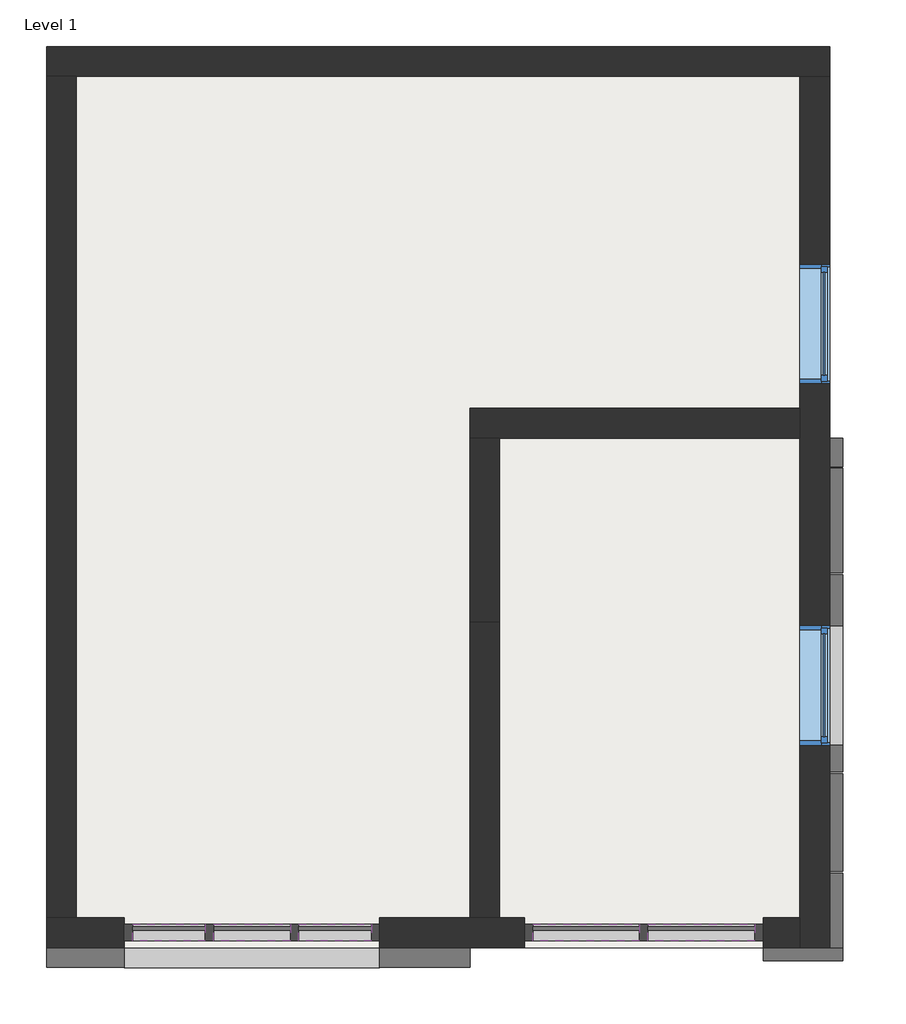
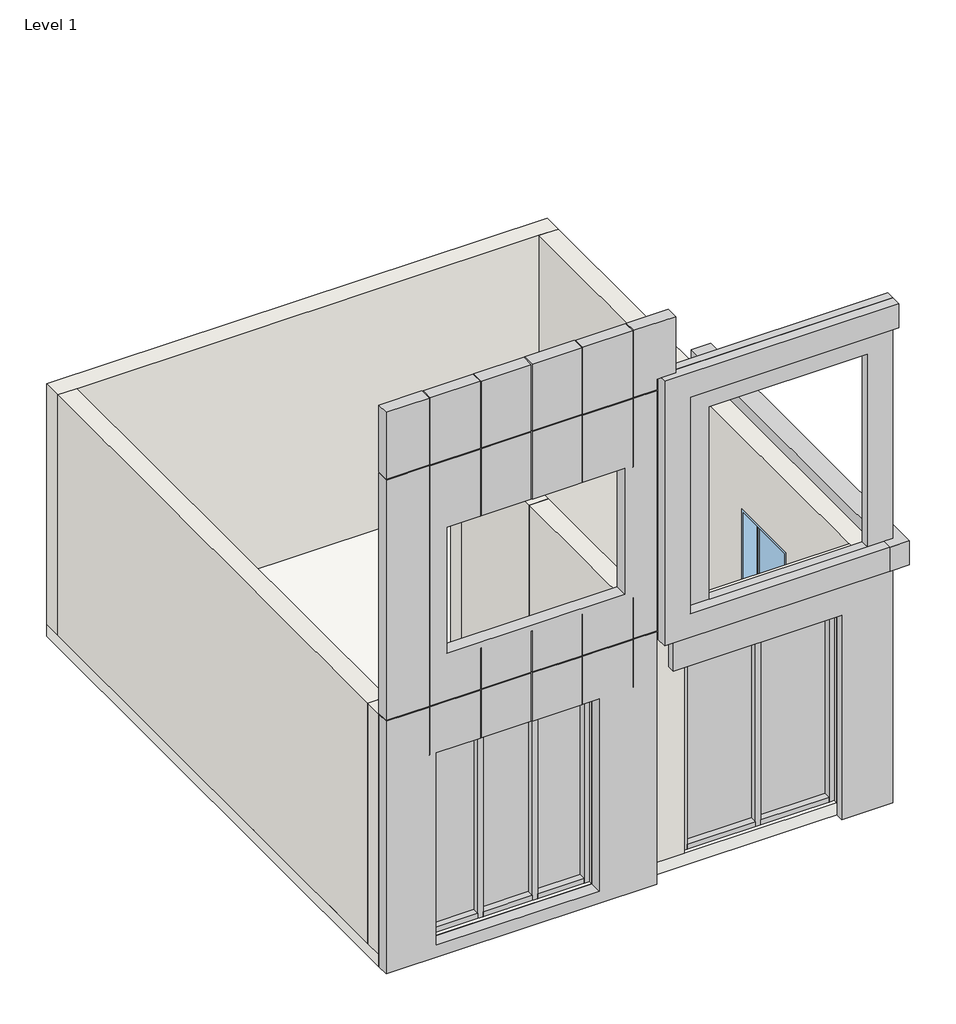
# One storey: 17 members, 7 walls, 5 plates, 2 windows, 1 proxy, 1 slab.
"""IFC4 building model written with IfcOpenShell, lengths in millimetres."""

from ifc_helpers import new_model, si_unit, frame, origin, origin_with_axes, place, context, project, spatial, polyline, outline, extrude, faceted_brep, transform, mapped, element, save
from components import generic_models_2_generic_models_2_1e037190, member_f0fea5a5, member_ee409385, member_c17f1be2, member_b26d3c89, member_9202991e, system_panel_glazed_061c0ed8, system_panel_glazed_2536b6f7, system_panel_glazed_348cf8e9, window_c1f32544, fixed_7_window_d95a62fe

model = new_model("IFC4")

# Units and contexts
model_context = context("Model", 3, world=origin())
ifc_project = project(units=[si_unit("LENGTHUNIT", "METRE", prefix="MILLI")], contexts=[model_context])

# Site, building, storey
site = spatial("IfcSite", under=ifc_project)
building = spatial("IfcBuilding", under=site)
storey = spatial("IfcBuildingStorey", under=building, Name="Level 1", Elevation=0.0)

# Proxy
placement = place(None, origin())
generic_models_2_generic_models_2_shape = generic_models_2_generic_models_2_1e037190(model_context)
element("IfcBuildingElementProxy", 1, Name="Generic Models 2 : Generic Models 2", ObjectType="Generic Models 2 : Generic Models 2", at=placement, inside=storey, context=model_context, shape_type="MappedRepresentation", body=[
    mapped(generic_models_2_generic_models_2_shape, transform((0.0, 0.0, 0.0), x_axis=(1.0, 0.0, 0.0), y_axis=(0.0, 1.0, 0.0), z_axis=(0.0, 0.0, 1.0))),
])

# Members
member_shape = member_f0fea5a5(model_context)
element("IfcMember", 2, ObjectType="Rectangular Mullion : 2.5\" x 5\" rectangular", at=placement, inside=storey, context=model_context, shape_type="MappedRepresentation", body=[
    mapped(member_shape, transform((-8698.6297584, 854.4262137, 0.0), x_axis=(1.0, 0.0, 0.0), y_axis=(0.0, -1.0, 0.0), z_axis=(0.0, 0.0, -1.0))),
])
element("IfcMember", 3, ObjectType="Rectangular Mullion : 2.5\" x 5\" rectangular", at=placement, inside=storey, context=model_context, shape_type="MappedRepresentation", body=[
    mapped(member_shape, transform((-12026.1620499, 854.4262137, 0.0), x_axis=(1.0, 0.0, 0.0), y_axis=(0.0, -1.0, 0.0), z_axis=(0.0, 0.0, -1.0))),
])
element("IfcMember", 4, ObjectType="Rectangular Mullion : 2.5\" x 5\" rectangular", at=placement, inside=storey, context=model_context, shape_type="MappedRepresentation", body=[
    mapped(member_shape, transform((-11374.2287168, 854.4262137, 0.0), x_axis=(1.0, 0.0, 0.0), y_axis=(0.0, -1.0, 0.0), z_axis=(0.0, 0.0, -1.0))),
])
member_2_shape = member_ee409385(model_context)
element("IfcMember", 5, ObjectType="Rectangular Mullion : 2.5\" x 5\" rectangular", at=placement, inside=storey, context=model_context, shape_type="MappedRepresentation", body=[
    mapped(member_2_shape, transform((-7784.2297584, 854.4262137, 0.0), x_axis=(1.0, 0.0, 0.0), y_axis=(0.0, -1.0, 0.0), z_axis=(0.0, 0.0, -1.0))),
])
element("IfcMember", 6, ObjectType="Rectangular Mullion : 2.5\" x 5\" rectangular", at=placement, inside=storey, context=model_context, shape_type="MappedRepresentation", body=[
    mapped(member_2_shape, transform((-10722.2953834, 854.4262137, 0.0), x_axis=(1.0, 0.0, 0.0), y_axis=(0.0, -1.0, 0.0), z_axis=(0.0, 0.0, -1.0))),
])
element("IfcMember", 7, ObjectType="Rectangular Mullion : 2.5\" x 5\" rectangular", at=placement, inside=storey, context=model_context, shape_type="MappedRepresentation", body=[
    mapped(member_2_shape, transform((-9613.0297584, 854.4262137, 2438.4), x_axis=(-1.0, 0.0, 0.0), y_axis=(0.0, -1.0, 0.0), z_axis=(0.0, 0.0, 1.0))),
])
element("IfcMember", 8, ObjectType="Rectangular Mullion : 2.5\" x 5\" rectangular", at=placement, inside=storey, context=model_context, shape_type="MappedRepresentation", body=[
    mapped(member_2_shape, transform((-12678.0953834, 854.4262137, 2438.4), x_axis=(-1.0, 0.0, 0.0), y_axis=(0.0, -1.0, 0.0), z_axis=(0.0, 0.0, 1.0))),
])
member_3_shape = member_c17f1be2(model_context)
element("IfcMember", 9, ObjectType="Rectangular Mullion : 2.5\" x 5\" rectangular", at=placement, inside=storey, context=model_context, shape_type="MappedRepresentation", body=[
    mapped(member_3_shape, transform((-7847.7297584, 854.4262137, 2438.4), x_axis=(0.0, 0.0, 1.0), y_axis=(0.0, -1.0, 0.0), z_axis=(1.0, 0.0, 0.0))),
])
element("IfcMember", 10, ObjectType="Rectangular Mullion : 2.5\" x 5\" rectangular", at=placement, inside=storey, context=model_context, shape_type="MappedRepresentation", body=[
    mapped(member_3_shape, transform((-8730.3797584, 854.4262137, 2438.4), x_axis=(0.0, 0.0, 1.0), y_axis=(0.0, -1.0, 0.0), z_axis=(1.0, 0.0, 0.0))),
])
element("IfcMember", 11, ObjectType="Rectangular Mullion : 2.5\" x 5\" rectangular", at=placement, inside=storey, context=model_context, shape_type="MappedRepresentation", body=[
    mapped(member_3_shape, transform((-9549.5297584, 854.4262137, 0.0), x_axis=(0.0, 0.0, -1.0), y_axis=(0.0, -1.0, 0.0), z_axis=(-1.0, 0.0, 0.0))),
])
element("IfcMember", 12, ObjectType="Rectangular Mullion : 2.5\" x 5\" rectangular", at=placement, inside=storey, context=model_context, shape_type="MappedRepresentation", body=[
    mapped(member_3_shape, transform((-8666.8797584, 854.4262137, 0.0), x_axis=(0.0, 0.0, -1.0), y_axis=(0.0, -1.0, 0.0), z_axis=(-1.0, 0.0, 0.0))),
])
member_4_shape = member_b26d3c89(model_context)
element("IfcMember", 13, ObjectType="Rectangular Mullion : 2.5\" x 5\" rectangular", at=placement, inside=storey, context=model_context, shape_type="MappedRepresentation", body=[
    mapped(member_4_shape, transform((-10785.7953834, 854.4262137, 2438.4), x_axis=(0.0, 0.0, 1.0), y_axis=(0.0, -1.0, 0.0), z_axis=(1.0, 0.0, 0.0))),
])
element("IfcMember", 14, ObjectType="Rectangular Mullion : 2.5\" x 5\" rectangular", at=placement, inside=storey, context=model_context, shape_type="MappedRepresentation", body=[
    mapped(member_4_shape, transform((-12057.9120499, 854.4262137, 2438.4), x_axis=(0.0, 0.0, 1.0), y_axis=(0.0, -1.0, 0.0), z_axis=(1.0, 0.0, 0.0))),
])
element("IfcMember", 15, ObjectType="Rectangular Mullion : 2.5\" x 5\" rectangular", at=placement, inside=storey, context=model_context, shape_type="MappedRepresentation", body=[
    mapped(member_4_shape, transform((-12614.5953834, 854.4262137, 0.0), x_axis=(0.0, 0.0, -1.0), y_axis=(0.0, -1.0, 0.0), z_axis=(-1.0, 0.0, 0.0))),
])
element("IfcMember", 16, ObjectType="Rectangular Mullion : 2.5\" x 5\" rectangular", at=placement, inside=storey, context=model_context, shape_type="MappedRepresentation", body=[
    mapped(member_4_shape, transform((-11342.4787168, 854.4262137, 0.0), x_axis=(0.0, 0.0, -1.0), y_axis=(0.0, -1.0, 0.0), z_axis=(-1.0, 0.0, 0.0))),
])
member_5_shape = member_9202991e(model_context)
element("IfcMember", 17, ObjectType="Rectangular Mullion : 2.5\" x 5\" rectangular", at=placement, inside=storey, context=model_context, shape_type="MappedRepresentation", body=[
    mapped(member_5_shape, transform((-11994.4120499, 854.4262137, 0.0), x_axis=(0.0, 0.0, -1.0), y_axis=(0.0, -1.0, 0.0), z_axis=(-1.0, 0.0, 0.0))),
])
element("IfcMember", 18, ObjectType="Rectangular Mullion : 2.5\" x 5\" rectangular", at=placement, inside=storey, context=model_context, shape_type="MappedRepresentation", body=[
    mapped(member_5_shape, transform((-11405.9787168, 854.4262137, 2438.4), x_axis=(0.0, 0.0, 1.0), y_axis=(0.0, -1.0, 0.0), z_axis=(1.0, 0.0, 0.0))),
])

# Plates
system_panel_glazed_shape = system_panel_glazed_061c0ed8(model_context)
element("IfcPlate", 19, ObjectType="System Panel : Glazed", at=placement, inside=storey, context=model_context, shape_type="MappedRepresentation", body=[
    mapped(system_panel_glazed_shape, transform((-9139.9547584, 854.4262137, 63.5), x_axis=(1.0, 0.0, 0.0), y_axis=(0.0, 1.0, 0.0), z_axis=(0.0, 0.0, 1.0))),
])
element("IfcPlate", 20, ObjectType="System Panel : Glazed", at=placement, inside=storey, context=model_context, shape_type="MappedRepresentation", body=[
    mapped(system_panel_glazed_shape, transform((-8257.3047584, 854.4262137, 63.5), x_axis=(1.0, 0.0, 0.0), y_axis=(0.0, 1.0, 0.0), z_axis=(0.0, 0.0, 1.0))),
])
system_panel_glazed_2_shape = system_panel_glazed_2536b6f7(model_context)
element("IfcPlate", 21, ObjectType="System Panel : Glazed", at=placement, inside=storey, context=model_context, shape_type="MappedRepresentation", body=[
    mapped(system_panel_glazed_2_shape, transform((-12336.2537167, 854.4262137, 63.5), x_axis=(1.0, 0.0, 0.0), y_axis=(0.0, 1.0, 0.0), z_axis=(0.0, 0.0, 1.0))),
])
element("IfcPlate", 22, ObjectType="System Panel : Glazed", at=placement, inside=storey, context=model_context, shape_type="MappedRepresentation", body=[
    mapped(system_panel_glazed_2_shape, transform((-11064.1370501, 854.4262137, 63.5), x_axis=(1.0, 0.0, 0.0), y_axis=(0.0, 1.0, 0.0), z_axis=(0.0, 0.0, 1.0))),
])
system_panel_glazed_3_shape = system_panel_glazed_348cf8e9(model_context)
element("IfcPlate", 23, ObjectType="System Panel : Glazed", at=placement, inside=storey, context=model_context, shape_type="MappedRepresentation", body=[
    mapped(system_panel_glazed_3_shape, transform((-11700.1953834, 854.4262137, 63.5), x_axis=(1.0, 0.0, 0.0), y_axis=(0.0, 1.0, 0.0), z_axis=(0.0, 0.0, 1.0))),
])

# Slab
element("IfcSlab", 24, ObjectType="6\" floor", at=placement, inside=storey, context=model_context, shape_type="SweptSolid", body=[
    extrude(outline(polyline([(-7274.9953834, 7640.1262137), (-7274.9953834, 740.1262137), (-13274.9953834, 740.1262137), (-13274.9953834, 7640.1262137), (-7274.9953834, 7640.1262137)])), frame((0.0, 0.0, -152.4), z_axis=(0.0, 0.0, 1.0), x_axis=(1.0, 0.0, 0.0)), (0.0, 0.0, 1.0), 152.4),
])

# Walls
element("IfcWall", 25, ObjectType="9\" wall", at=placement, inside=storey, context=model_context, shape_type="Brep", body=[
    faceted_brep([(-13274.9953834, 7411.5262137, 0.0), (-13046.3953834, 7411.5262137, 0.0), (-7503.5953834, 7411.5262137, 0.0), (-7274.9953834, 7411.5262137, 0.0), (-7274.9953834, 7411.5262137, 3048.0), (-7503.5953834, 7411.5262137, 3048.0), (-13046.3953834, 7411.5262137, 3048.0), (-13274.9953834, 7411.5262137, 3048.0), (-13274.9953834, 7640.1262137, 0.0), (-13274.9953834, 7640.1262137, 3048.0), (-7274.9953834, 7640.1262137, 3048.0), (-7274.9953834, 7640.1262137, 0.0)], [[[0, 1, 2, 3, 4, 5, 6, 7]], [[8, 9, 10, 11]], [[3, 2, 1, 0, 8, 11]], [[7, 6, 5, 4, 10, 9]], [[4, 3, 11, 10]], [[0, 7, 9, 8]]]),
])
element("IfcWall", 26, ObjectType="9\" wall", at=placement, inside=storey, context=model_context, shape_type="Brep", body=[
    faceted_brep([(-7503.5953834, 740.1262137, 3048.0), (-7503.5953834, 968.7262137, 3048.0), (-7503.5953834, 4640.1176199, 3048.0), (-7503.5953834, 4868.7176199, 3048.0), (-7503.5953834, 7411.5262137, 3048.0), (-7503.5953834, 7411.5262137, 0.0), (-7503.5953834, 4868.7176199, 0.0), (-7503.5953834, 4640.1176199, 0.0), (-7503.5953834, 3205.0176199, 0.0), (-7503.5953834, 3205.0176199, 2133.6), (-7503.5953834, 2290.6176199, 2133.6), (-7503.5953834, 2290.6176199, 0.0), (-7503.5953834, 968.7262137, 0.0), (-7503.5953834, 740.1262137, 0.0), (-7503.5953834, 5059.2176199, 2133.6), (-7503.5953834, 5059.2176199, 914.4), (-7503.5953834, 5973.6176199, 914.4), (-7503.5953834, 5973.6176199, 2133.6), (-7274.9953834, 7411.5262137, 3048.0), (-7274.9953834, 740.1262137, 3048.0), (-7274.9953834, 740.1262137, 0.0), (-7274.9953834, 2290.6176199, 0.0), (-7274.9953834, 2290.6176199, 2133.6), (-7274.9953834, 3205.0176199, 2133.6), (-7274.9953834, 3205.0176199, 0.0), (-7274.9953834, 7411.5262137, 0.0), (-7274.9953834, 5059.2176199, 2133.6), (-7274.9953834, 5973.6176199, 2133.6), (-7274.9953834, 5973.6176199, 914.4), (-7274.9953834, 5059.2176199, 914.4)], [[[0, 1, 2, 3, 4, 5, 6, 7, 8, 9, 10, 11, 12, 13], [14, 15, 16, 17]], [[18, 19, 20, 21, 22, 23, 24, 25], [26, 27, 28, 29]], [[5, 25, 24, 8, 7, 6]], [[20, 13, 12, 11, 21]], [[4, 3, 2, 1, 0, 19, 18]], [[5, 4, 18, 25]], [[0, 13, 20, 19]], [[15, 14, 26, 29]], [[16, 15, 29, 28]], [[17, 16, 28, 27]], [[14, 17, 27, 26]], [[10, 22, 21, 11]], [[23, 9, 8, 24]], [[22, 10, 9, 23]]]),
])
element("IfcWall", 27, ObjectType="9\" wall", at=placement, inside=storey, context=model_context, shape_type="Brep", body=[
    faceted_brep([(-13274.9953834, 968.7262137, 3048.0), (-13046.3953834, 968.7262137, 3048.0), (-10032.1297584, 968.7262137, 3048.0), (-9803.5297584, 968.7262137, 3048.0), (-7503.5953834, 968.7262137, 3048.0), (-7503.5953834, 968.7262137, 0.0), (-7784.2297584, 968.7262137, 0.0), (-7784.2297584, 968.7262137, 2438.4), (-9613.0297584, 968.7262137, 2438.4), (-9613.0297584, 968.7262137, 0.0), (-9803.5297584, 968.7262137, 0.0), (-10032.1297584, 968.7262137, 0.0), (-10722.2953834, 968.7262137, 0.0), (-10722.2953834, 968.7262137, 2438.4), (-12678.0953834, 968.7262137, 2438.4), (-12678.0953834, 968.7262137, 0.0), (-13046.3953834, 968.7262137, 0.0), (-13274.9953834, 968.7262137, 0.0), (-7503.5953834, 740.1262137, 3048.0), (-13274.9953834, 740.1262137, 3048.0), (-13274.9953834, 740.1262137, 0.0), (-12678.0953834, 740.1262137, 0.0), (-12678.0953834, 740.1262137, 2438.4), (-10722.2953834, 740.1262137, 2438.4), (-10722.2953834, 740.1262137, 0.0), (-9613.0297584, 740.1262137, 0.0), (-9613.0297584, 740.1262137, 2438.4), (-7784.2297584, 740.1262137, 2438.4), (-7784.2297584, 740.1262137, 0.0), (-7503.5953834, 740.1262137, 0.0)], [[[0, 1, 2, 3, 4, 5, 6, 7, 8, 9, 10, 11, 12, 13, 14, 15, 16, 17]], [[18, 19, 20, 21, 22, 23, 24, 25, 26, 27, 28, 29]], [[5, 29, 28, 6]], [[20, 17, 16, 15, 21]], [[9, 25, 24, 12, 11, 10]], [[4, 3, 2, 1, 0, 19, 18]], [[5, 4, 18, 29]], [[0, 17, 20, 19]], [[8, 26, 25, 9]], [[26, 8, 7, 27]], [[27, 7, 6, 28]], [[14, 22, 21, 15]], [[22, 14, 13, 23]], [[23, 13, 12, 24]]]),
])
element("IfcWall", 28, ObjectType="9\" wall", at=placement, inside=storey, context=model_context, shape_type="SweptSolid", body=[
    extrude(outline(polyline([(-13046.3953834, 7411.5262137), (-13046.3953834, 968.7262137), (-13274.9953834, 968.7262137), (-13274.9953834, 7411.5262137), (-13046.3953834, 7411.5262137)])), origin_with_axes(), (0.0, 0.0, 1.0), 3048.0),
])
element("IfcWall", 29, ObjectType="9\" wall", at=placement, inside=storey, context=model_context, shape_type="Brep", body=[
    faceted_brep([(-7503.5953834, 4868.7176199, 0.0), (-10032.1297584, 4868.7176199, 0.0), (-10032.1297584, 4868.7176199, 3048.0), (-7503.5953834, 4868.7176199, 3048.0), (-7503.5953834, 4640.1176199, 0.0), (-7503.5953834, 4640.1176199, 3048.0), (-9803.5297584, 4640.1176199, 3048.0), (-10032.1297584, 4640.1176199, 3048.0), (-10032.1297584, 4640.1176199, 0.0), (-9803.5297584, 4640.1176199, 0.0)], [[[0, 1, 2, 3]], [[4, 5, 6, 7, 8, 9]], [[1, 0, 4, 9, 8]], [[3, 2, 7, 6, 5]], [[0, 3, 5, 4]], [[2, 1, 8, 7]]]),
])
element("IfcWall", 30, ObjectType="9\" wall", at=placement, inside=storey, context=model_context, shape_type="SweptSolid", body=[
    extrude(outline(polyline([(-10032.1297584, 3230.4176199), (-10032.1297584, 4640.1176199), (-9803.5297584, 4640.1176199), (-9803.5297584, 3230.4176199), (-10032.1297584, 3230.4176199)])), origin_with_axes(), (0.0, 0.0, 1.0), 3048.0),
])
element("IfcWall", 31, ObjectType="9\" wall", at=placement, inside=storey, context=model_context, shape_type="SweptSolid", body=[
    extrude(outline(polyline([(-10032.1297584, 968.7262137), (-10032.1297584, 3230.4176199), (-9803.5297584, 3230.4176199), (-9803.5297584, 968.7262137), (-10032.1297584, 968.7262137)])), origin_with_axes(), (0.0, 0.0, 1.0), 3048.0),
])

# Windows
window_shape = window_c1f32544(model_context)
element("IfcWindow", 32, ObjectType="Fixed : 36\" x 48\"", at=placement, inside=storey, context=model_context, shape_type="MappedRepresentation", body=[
    mapped(window_shape, transform((-7389.2953834, 5478.3176199, 0.0), x_axis=(0.0, -1.0, 0.0), y_axis=(1.0, 0.0, 0.0), z_axis=(0.0, 0.0, 1.0))),
])
fixed_7_window_shape = fixed_7_window_d95a62fe(model_context)
element("IfcWindow", 33, ObjectType="Fixed : 7' window", at=placement, inside=storey, context=model_context, shape_type="MappedRepresentation", body=[
    mapped(fixed_7_window_shape, transform((-7389.2953834, 2709.7176199, -914.4), x_axis=(0.0, -1.0, 0.0), y_axis=(1.0, 0.0, 0.0), z_axis=(0.0, 0.0, 1.0))),
])

save(model, "model.ifc")

# Revit data of these elements
# Type "Rectangular Mullion : 2.5\" x 5\" rectangular"
#   built-in parameter 1007304 = 0.416667 (stored number, unit not read)
#   built-in parameter 1007301 = 0.104167 (stored number, unit not read)
#   built-in parameter 1007300 = 0.104167 (stored number, unit not read)
# Type "System Panel : Glazed"
#   Construction Type Id = "GSP4R"
#   Analytic Construction = "1/8 in Pilkington single glazing"
#   Visual Light Transmittance = 0.9
#   Solar Heat Gain Coefficient = 0.86
#   Heat Transfer Coefficient (U) = 1.18115 BTU/(h·ft²·°F)
#   Define Thermal Properties by = 1
# Type "6\" floor"
#   Assembly Code = "B1010"
#   Function = 0
#   Layers, outside or top first: 0' - 6" no material (function 1)
# Type "9\" wall"
#   Assembly Code = "B2010"
#   Layers, outside or top first: 0' - 9" "Asphalt, Pavement, Light Grey" (function 1)
# Type "Fixed : 36\" x 48\""
#   Type Mark = "1"
#   Construction Type Id = "GSP4R"
#   Assembly Code = "B2020100"
#   Analytic Construction = "1/8 in Pilkington single glazing"
#   Visual Light Transmittance = 0.9
#   Solar Heat Gain Coefficient = 0.78
#   Heat Transfer Coefficient (U) = 0.6496 BTU/(h·ft²·°F)
#   Height = 4' - 0"
#   Default Sill Height = 3' - 0"
#   Width = 3' - 0"
#   Window Inset = 0' - 0 3/4"
#   Define Thermal Properties by = 1
#   Define Thermal Properties by = 1
#   Glass Pane Material = Glass
#   Sash Material = Sash
#   Wall Closure = (empty or 0)
# Type "Fixed : 7' window"
#   Type Mark = "18"
#   Construction Type Id = "GSP4R"
#   Assembly Code = "B2020100"
#   Analytic Construction = "1/8 in Pilkington single glazing"
#   Visual Light Transmittance = 0.9
#   Solar Heat Gain Coefficient = 0.78
#   Heat Transfer Coefficient (U) = 0.6496 BTU/(h·ft²·°F)
#   Height = 7' - 0"
#   Default Sill Height = 3' - 0"
#   Width = 3' - 0"
#   Window Inset = 0' - 0 3/4"
#   Define Thermal Properties by = 1
#   Glass Pane Material = Glass
#   Sash Material = Sash
#   Wall Closure = (empty or 0)
# Element 1 (IfcBuildingElementProxy, "Generic Models 2 : Generic Models 2")
#   Phase Created = New Construction
#   Materials on its faces: "Damp-proofing", "Asphalt, Pavement, Light Grey"
# Elements 2, 3, 4, 5, 6, 7, 8, 9, 10, 11, 12, 13, 14, 15, 16, 17, 18 (IfcMember, "Rectangular Mullion : 2.5\" x 5\" rectangular")
#   Phase Created = New Construction
#   Materials on its faces: "Aluminum"
# Elements 19, 20, 21, 22, 23 (IfcPlate, "System Panel : Glazed")
#   Phase Created = New Construction
#   Materials on its faces: "Glass"
# Element 24 (IfcSlab, "6\" floor")
#   Height Offset From Level = 0' - 0"
#   Phase Created = New Construction
#   Materials on its faces: "Default Floor"
# Elements 25, 26, 27, 28, 29, 30, 31 (IfcWall, "9\" wall")
#   Top Offset = 0' - 0"
#   Base Offset = 0' - 0"
#   wall height = 10' - 0"
#   Phase Created = New Construction
#   Base Constraint = Level 1
#   Top Constraint = Level 2
#   Materials on its faces: "Asphalt, Pavement, Light Grey"
# Element 32 (IfcWindow, "Fixed : 36\" x 48\"")
#   Mark = "1"
#   Phase Created = New Construction
#   Materials on its faces: "Sash", "Glass"
# Element 33 (IfcWindow, "Fixed : 7' window")
#   Mark = "3"
#   Phase Created = New Construction
#   Materials on its faces: "Sash", "Glass"
# Materials
#   "Asphalt, Pavement, Light Grey": class "Generic", colour RGB 120 120 120, transparency 0, Description = "Asphalt or tarmac paving", Cost = 0
#   "Glass": class "Glass", colour RGB 0 128 192, transparency 0.75, Description = "Soda Lime Glass", Cost = 0
#   "Sash": class "Wood", colour RGB 224 178 126, transparency 0, Cost = 0
#   "Damp-proofing": class "Generic", colour RGB 127 127 127, transparency 0, Description = "Damp-proofing", Cost = 0
#   "Aluminum": class "Metal", colour RGB 247 247 247, transparency 0, Description = "Aluminum 6061", Cost = 0
#   "Default Floor": colour RGB 128 128 128, transparency 0, Cost = 0
